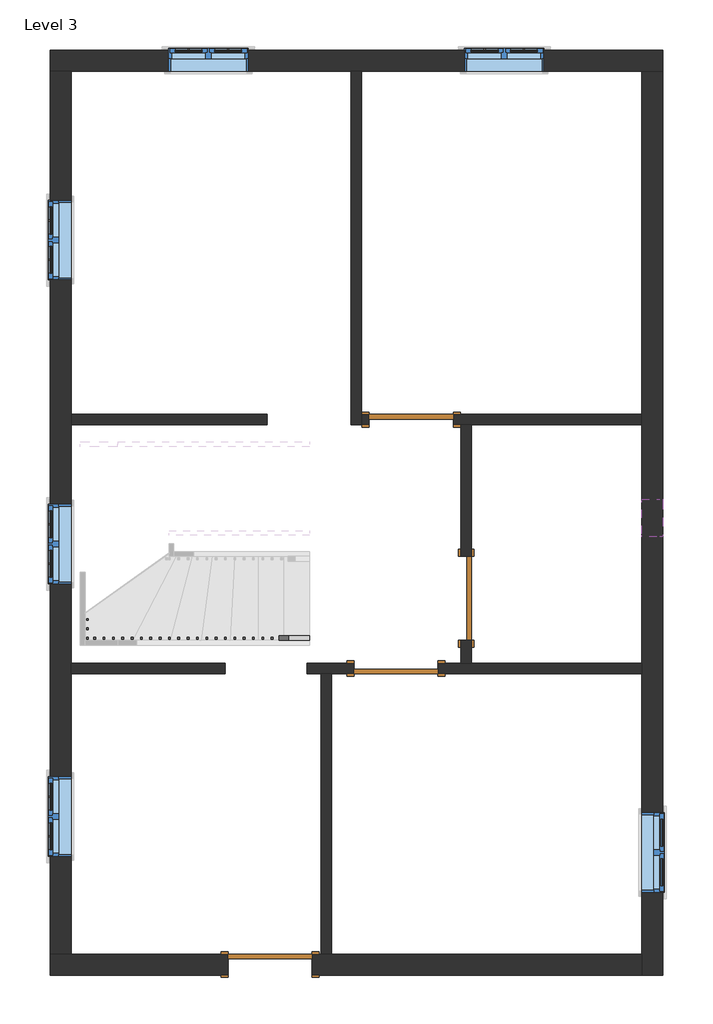
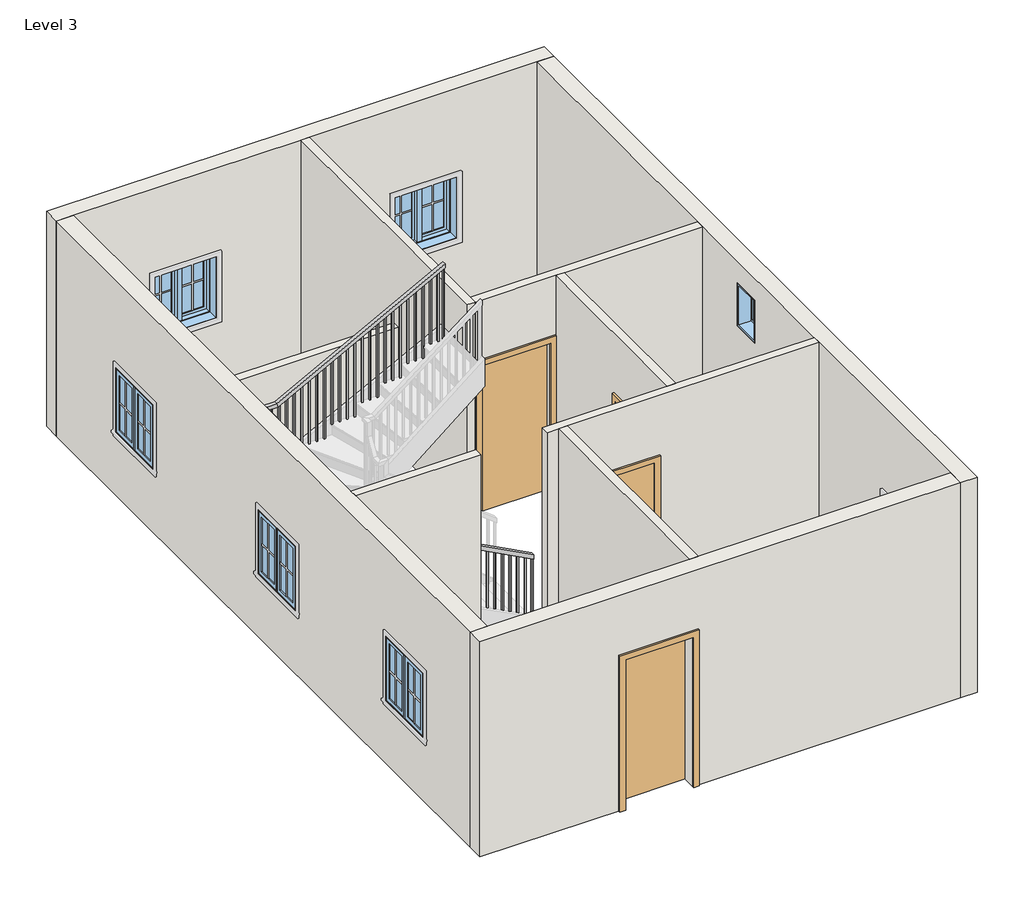
# One storey, part 1 of 2: 11 walls, 7 windows, 4 doors, 1 railing.
"""IFC4 building model written with IfcOpenShell, lengths in millimetres."""

from ifc_helpers import new_model, si_unit, frame, origin, place, context, project, spatial, polyline, outline, extrude, faceted_brep, transform, mapped, element, save
from components import door_e5f9f3c4, door_305aa2a5, door_a90ba1ad, window_aa618e30, window_339605e1

model = new_model("IFC4")

# Units and contexts
model_context = context("Model", 3, world=origin())
ifc_project = project(units=[si_unit("LENGTHUNIT", "METRE", prefix="MILLI")], contexts=[model_context])

# Site, building, storey
site = spatial("IfcSite", under=ifc_project)
building = spatial("IfcBuilding", under=site)
storey = spatial("IfcBuildingStorey", under=building, Name="Level 3", Elevation=3200.4)

# Doors
placement = place(None, origin())
door_shape = door_e5f9f3c4(model_context)
element("IfcDoor", 1, ObjectType="Single-Flush : 36\" x 84\"", at=placement, inside=storey, context=model_context, shape_type="MappedRepresentation", body=[
    mapped(door_shape, transform((-78.9949167, -802.9070853, 3200.4), x_axis=(0.0, -1.0, 0.0), y_axis=(1.0, 0.0, 0.0), z_axis=(0.0, 0.0, 1.0))),
])
element("IfcDoor", 2, ObjectType="Single-Flush : 36\" x 84\"", at=placement, inside=storey, context=model_context, shape_type="MappedRepresentation", body=[
    mapped(door_shape, transform((-840.9949167, -1564.9070853, 3200.4), x_axis=(-1.0, 0.0, 0.0), y_axis=(0.0, -1.0, 0.0), z_axis=(0.0, 0.0, 1.0))),
])
door_2_shape = door_305aa2a5(model_context)
element("IfcDoor", 3, ObjectType="Single-Flush : 36\" x 84\"", at=placement, inside=storey, context=model_context, shape_type="MappedRepresentation", body=[
    mapped(door_2_shape, transform((-675.8949167, 1140.1929147, 3200.4), x_axis=(-1.0, 0.0, 0.0), y_axis=(0.0, -1.0, 0.0), z_axis=(0.0, 0.0, 1.0))),
])
door_3_shape = door_a90ba1ad(model_context)
element("IfcDoor", 4, ObjectType="Single-Flush : 36\" x 84\"", at=placement, inside=storey, context=model_context, shape_type="MappedRepresentation", body=[
    mapped(door_3_shape, transform((-2212.5949167, -4784.3570853, 3200.4), x_axis=(-1.0, 0.0, 0.0), y_axis=(0.0, -1.0, 0.0), z_axis=(0.0, 0.0, 1.0))),
])

# Railing
element("IfcRailing", 5, ObjectType="Handrail - Rectangular", at=placement, inside=storey, context=model_context, shape_type="SolidModel", body=[
    faceted_brep([(-1783.4132248, -1260.1070853, 4284.1333333), (-1783.4132248, -1260.1070853, 4226.6742652), (-1783.4132248, -1209.3070853, 4226.6742652), (-1783.4132248, -1209.3070853, 4284.1333333), (-4041.1382869, -1260.1070853, 5477.4239201), (-4053.7373514, -1260.1070853, 5426.6239201), (-4053.7373514, -1209.3070853, 5426.6239201), (-4041.1382869, -1209.3070853, 5477.4239201), (-4225.5449167, -1260.1070853, 5477.4239201), (-4225.5449167, -1260.1070853, 5426.6239201), (-4174.7449167, -1209.3070853, 5426.6239201), (-4174.7449167, -1209.3070853, 5477.4239201), (-4225.5449167, -972.7952032, 5477.4239201), (-4225.5449167, -964.8446271, 5426.6239201), (-4174.7449167, -964.8446271, 5426.6239201), (-4174.7449167, -972.7952032, 5477.4239201), (-4225.5449167, 560.7810325, 5969.5094132), (-4225.5449167, 568.7316087, 5918.7094132), (-4174.7449167, 568.7316087, 5918.7094132), (-4174.7449167, 560.7810325, 5969.5094132), (-4225.5449167, 848.0929147, 5969.5094132), (-4225.5449167, 848.0929147, 5918.7094132), (-4174.7449167, 797.2929147, 5918.7094132), (-4174.7449167, 797.2929147, 5969.5094132), (-4041.1382869, 848.0929147, 5969.5094132), (-4028.5392223, 848.0929147, 5918.7094132), (-4028.5392223, 797.2929147, 5918.7094132), (-4041.1382869, 797.2929147, 5969.5094132), (-1783.4132248, 848.0929147, 7162.8), (-1783.4132248, 797.2929147, 7162.8), (-1783.4132248, 797.2929147, 7105.3409318), (-1783.4132248, 848.0929147, 7105.3409318)], [[[0, 1, 2, 3]], [[1, 0, 4, 5]], [[2, 1, 5, 6]], [[3, 2, 6, 7]], [[0, 3, 7, 4]], [[5, 4, 8, 9]], [[6, 5, 9, 10]], [[7, 6, 10, 11]], [[4, 7, 11, 8]], [[9, 8, 12, 13]], [[10, 9, 13, 14]], [[11, 10, 14, 15]], [[8, 11, 15, 12]], [[13, 12, 16, 17]], [[14, 13, 17, 18]], [[15, 14, 18, 19]], [[12, 15, 19, 16]], [[17, 16, 20, 21]], [[18, 17, 21, 22]], [[19, 18, 22, 23]], [[16, 19, 23, 20]], [[21, 20, 24, 25]], [[22, 21, 25, 26]], [[23, 22, 26, 27]], [[20, 23, 27, 24]], [[28, 29, 30, 31]], [[25, 24, 28, 31]], [[26, 25, 31, 30]], [[27, 26, 30, 29]], [[24, 27, 29, 28]]]),
    extrude(outline(polyline([(7058.0597858, -1872.8699167), (6079.0666667, -1872.8699167), (6079.0666667, -1853.8199167), (7068.1284102, -1853.8199167), (7058.0597858, -1872.8699167)])), frame((0.0, 813.1679147, 0.0), z_axis=(0.0, 1.0, 0.0), x_axis=(0.0, 0.0, 1.0)), (0.0, 0.0, 1.0), 19.05),
    extrude(outline(polyline([(7004.3604556, -1974.4699167), (6079.0666667, -1974.4699167), (6079.0666667, -1955.4199167), (7014.42908, -1955.4199167), (7004.3604556, -1974.4699167)])), frame((0.0, 813.1679147, 0.0), z_axis=(0.0, 1.0, 0.0), x_axis=(0.0, 0.0, 1.0)), (0.0, 0.0, 1.0), 19.05),
    extrude(outline(polyline([(6950.6611254, -2076.0699167), (5909.7333333, -2076.0699167), (5909.7333333, -2057.0199167), (6960.7297498, -2057.0199167), (6950.6611254, -2076.0699167)])), frame((0.0, 813.1679147, 0.0), z_axis=(0.0, 1.0, 0.0), x_axis=(0.0, 0.0, 1.0)), (0.0, 0.0, 1.0), 19.05),
    extrude(outline(polyline([(6896.9617952, -2177.6699167), (5909.7333333, -2177.6699167), (5909.7333333, -2158.6199167), (6907.0304196, -2158.6199167), (6896.9617952, -2177.6699167)])), frame((0.0, 813.1679147, 0.0), z_axis=(0.0, 1.0, 0.0), x_axis=(0.0, 0.0, 1.0)), (0.0, 0.0, 1.0), 19.05),
    extrude(outline(polyline([(6843.262465, -2279.2699167), (5909.7333333, -2279.2699167), (5909.7333333, -2260.2199167), (6853.3310894, -2260.2199167), (6843.262465, -2279.2699167)])), frame((0.0, 813.1679147, 0.0), z_axis=(0.0, 1.0, 0.0), x_axis=(0.0, 0.0, 1.0)), (0.0, 0.0, 1.0), 19.05),
    extrude(outline(polyline([(6789.5631348, -2380.8699167), (5740.4, -2380.8699167), (5740.4, -2361.8199167), (6799.6317592, -2361.8199167), (6789.5631348, -2380.8699167)])), frame((0.0, 813.1679147, 0.0), z_axis=(0.0, 1.0, 0.0), x_axis=(0.0, 0.0, 1.0)), (0.0, 0.0, 1.0), 19.05),
    extrude(outline(polyline([(6735.8638046, -2482.4699167), (5740.4, -2482.4699167), (5740.4, -2463.4199167), (6745.932429, -2463.4199167), (6735.8638046, -2482.4699167)])), frame((0.0, 813.1679147, 0.0), z_axis=(0.0, 1.0, 0.0), x_axis=(0.0, 0.0, 1.0)), (0.0, 0.0, 1.0), 19.05),
    extrude(outline(polyline([(6682.1644744, -2584.0699167), (5740.4, -2584.0699167), (5740.4, -2565.0199167), (6692.2330988, -2565.0199167), (6682.1644744, -2584.0699167)])), frame((0.0, 813.1679147, 0.0), z_axis=(0.0, 1.0, 0.0), x_axis=(0.0, 0.0, 1.0)), (0.0, 0.0, 1.0), 19.05),
    extrude(outline(polyline([(6628.4651442, -2685.6699167), (5571.0666667, -2685.6699167), (5571.0666667, -2666.6199167), (6638.5337686, -2666.6199167), (6628.4651442, -2685.6699167)])), frame((0.0, 813.1679147, 0.0), z_axis=(0.0, 1.0, 0.0), x_axis=(0.0, 0.0, 1.0)), (0.0, 0.0, 1.0), 19.05),
    extrude(outline(polyline([(6574.765814, -2787.2699167), (5571.0666667, -2787.2699167), (5571.0666667, -2768.2199167), (6584.8344384, -2768.2199167), (6574.765814, -2787.2699167)])), frame((0.0, 813.1679147, 0.0), z_axis=(0.0, 1.0, 0.0), x_axis=(0.0, 0.0, 1.0)), (0.0, 0.0, 1.0), 19.05),
    extrude(outline(polyline([(6521.0664838, -2888.8699167), (5571.0666667, -2888.8699167), (5571.0666667, -2869.8199167), (6531.1351082, -2869.8199167), (6521.0664838, -2888.8699167)])), frame((0.0, 813.1679147, 0.0), z_axis=(0.0, 1.0, 0.0), x_axis=(0.0, 0.0, 1.0)), (0.0, 0.0, 1.0), 19.05),
    extrude(outline(polyline([(6467.3671536, -2990.4699167), (5401.7333333, -2990.4699167), (5401.7333333, -2971.4199167), (6477.435778, -2971.4199167), (6467.3671536, -2990.4699167)])), frame((0.0, 813.1679147, 0.0), z_axis=(0.0, 1.0, 0.0), x_axis=(0.0, 0.0, 1.0)), (0.0, 0.0, 1.0), 19.05),
    extrude(outline(polyline([(6413.6678234, -3092.0699167), (5401.7333333, -3092.0699167), (5401.7333333, -3073.0199167), (6423.7364478, -3073.0199167), (6413.6678234, -3092.0699167)])), frame((0.0, 813.1679147, 0.0), z_axis=(0.0, 1.0, 0.0), x_axis=(0.0, 0.0, 1.0)), (0.0, 0.0, 1.0), 19.05),
    extrude(outline(polyline([(6359.9684932, -3193.6699167), (5401.7333333, -3193.6699167), (5401.7333333, -3174.6199167), (6370.0371176, -3174.6199167), (6359.9684932, -3193.6699167)])), frame((0.0, 813.1679147, 0.0), z_axis=(0.0, 1.0, 0.0), x_axis=(0.0, 0.0, 1.0)), (0.0, 0.0, 1.0), 19.05),
    extrude(outline(polyline([(6306.269163, -3295.2699167), (5401.7333333, -3295.2699167), (5401.7333333, -3276.2199167), (6316.3377874, -3276.2199167), (6306.269163, -3295.2699167)])), frame((0.0, 813.1679147, 0.0), z_axis=(0.0, 1.0, 0.0), x_axis=(0.0, 0.0, 1.0)), (0.0, 0.0, 1.0), 19.05),
    extrude(outline(polyline([(6252.5698328, -3396.8699167), (5232.4, -3396.8699167), (5232.4, -3377.8199167), (6262.6384572, -3377.8199167), (6252.5698328, -3396.8699167)])), frame((0.0, 813.1679147, 0.0), z_axis=(0.0, 1.0, 0.0), x_axis=(0.0, 0.0, 1.0)), (0.0, 0.0, 1.0), 19.05),
    extrude(outline(polyline([(6198.8705026, -3498.4699167), (5232.4, -3498.4699167), (5232.4, -3479.4199167), (6208.939127, -3479.4199167), (6198.8705026, -3498.4699167)])), frame((0.0, 813.1679147, 0.0), z_axis=(0.0, 1.0, 0.0), x_axis=(0.0, 0.0, 1.0)), (0.0, 0.0, 1.0), 19.05),
    extrude(outline(polyline([(6145.1711724, -3600.0699167), (5232.4, -3600.0699167), (5232.4, -3581.0199167), (6155.2397968, -3581.0199167), (6145.1711724, -3600.0699167)])), frame((0.0, 813.1679147, 0.0), z_axis=(0.0, 1.0, 0.0), x_axis=(0.0, 0.0, 1.0)), (0.0, 0.0, 1.0), 19.05),
    extrude(outline(polyline([(6091.4718422, -3701.6699167), (5232.4, -3701.6699167), (5232.4, -3682.6199167), (6101.5404666, -3682.6199167), (6091.4718422, -3701.6699167)])), frame((0.0, 813.1679147, 0.0), z_axis=(0.0, 1.0, 0.0), x_axis=(0.0, 0.0, 1.0)), (0.0, 0.0, 1.0), 19.05),
    extrude(outline(polyline([(6037.772512, -3803.2699167), (5063.0666667, -3803.2699167), (5063.0666667, -3784.2199167), (6047.8411364, -3784.2199167), (6037.772512, -3803.2699167)])), frame((0.0, 813.1679147, 0.0), z_axis=(0.0, 1.0, 0.0), x_axis=(0.0, 0.0, 1.0)), (0.0, 0.0, 1.0), 19.05),
    extrude(outline(polyline([(5984.0731818, -3904.8699167), (5063.0666667, -3904.8699167), (5063.0666667, -3885.8199167), (5994.1418062, -3885.8199167), (5984.0731818, -3904.8699167)])), frame((0.0, 813.1679147, 0.0), z_axis=(0.0, 1.0, 0.0), x_axis=(0.0, 0.0, 1.0)), (0.0, 0.0, 1.0), 19.05),
    extrude(outline(polyline([(5930.3738516, -4006.4699167), (5063.0666667, -4006.4699167), (5063.0666667, -3987.4199167), (5940.442476, -3987.4199167), (5930.3738516, -4006.4699167)])), frame((0.0, 813.1679147, 0.0), z_axis=(0.0, 1.0, 0.0), x_axis=(0.0, 0.0, 1.0)), (0.0, 0.0, 1.0), 19.05),
    extrude(outline(polyline([(-4108.0699167, 832.2179147), (-4089.0199167, 832.2179147), (-4089.0199167, 813.1679147), (-4108.0699167, 813.1679147), (-4108.0699167, 832.2179147)])), frame((0.0, 0.0, 5063.0666667), z_axis=(0.0, 0.0, 1.0), x_axis=(1.0, 0.0, 0.0)), (0.0, 0.0, 1.0), 855.6427466),
    extrude(outline(polyline([(-4209.6699167, 787.7679147), (-4209.6699167, 806.8179147), (-4190.6199167, 806.8179147), (-4190.6199167, 787.7679147), (-4209.6699167, 787.7679147)])), frame((0.0, 0.0, 5063.0666667), z_axis=(0.0, 0.0, 1.0), x_axis=(1.0, 0.0, 0.0)), (0.0, 0.0, 1.0), 855.6427466),
    extrude(outline(polyline([(-4209.6699167, 686.1679147), (-4209.6699167, 705.2179147), (-4190.6199167, 705.2179147), (-4190.6199167, 686.1679147), (-4209.6699167, 686.1679147)])), frame((0.0, 0.0, 5063.0666667), z_axis=(0.0, 0.0, 1.0), x_axis=(1.0, 0.0, 0.0)), (0.0, 0.0, 1.0), 855.6427466),
    extrude(outline(polyline([(-4209.6699167, 584.5679147), (-4209.6699167, 603.6179147), (-4190.6199167, 603.6179147), (-4190.6199167, 584.5679147), (-4209.6699167, 584.5679147)])), frame((0.0, 0.0, 5063.0666667), z_axis=(0.0, 0.0, 1.0), x_axis=(1.0, 0.0, 0.0)), (0.0, 0.0, 1.0), 855.6427466),
    extrude(outline(polyline([(502.0179147, 5897.3026907), (502.0179147, 4893.7333333), (482.9679147, 4893.7333333), (482.9679147, 5891.1900316), (502.0179147, 5897.3026907)])), frame((-4209.6699167, 0.0, 0.0), z_axis=(1.0, 0.0, 0.0), x_axis=(0.0, 1.0, 0.0)), (0.0, 0.0, 1.0), 19.05),
    extrude(outline(polyline([(400.4179147, 5864.7018425), (400.4179147, 4893.7333333), (381.3679147, 4893.7333333), (381.3679147, 5858.5891834), (400.4179147, 5864.7018425)])), frame((-4209.6699167, 0.0, 0.0), z_axis=(1.0, 0.0, 0.0), x_axis=(0.0, 1.0, 0.0)), (0.0, 0.0, 1.0), 19.05),
    extrude(outline(polyline([(298.8179147, 5832.1009942), (298.8179147, 4893.7333333), (279.7679147, 4893.7333333), (279.7679147, 5825.9883352), (298.8179147, 5832.1009942)])), frame((-4209.6699167, 0.0, 0.0), z_axis=(1.0, 0.0, 0.0), x_axis=(0.0, 1.0, 0.0)), (0.0, 0.0, 1.0), 19.05),
    extrude(outline(polyline([(197.2179147, 5799.500146), (197.2179147, 4893.7333333), (178.1679147, 4893.7333333), (178.1679147, 5793.387487), (197.2179147, 5799.500146)])), frame((-4209.6699167, 0.0, 0.0), z_axis=(1.0, 0.0, 0.0), x_axis=(0.0, 1.0, 0.0)), (0.0, 0.0, 1.0), 19.05),
    extrude(outline(polyline([(95.6179147, 5766.8992978), (95.6179147, 4893.7333333), (76.5679147, 4893.7333333), (76.5679147, 5760.7866387), (95.6179147, 5766.8992978)])), frame((-4209.6699167, 0.0, 0.0), z_axis=(1.0, 0.0, 0.0), x_axis=(0.0, 1.0, 0.0)), (0.0, 0.0, 1.0), 19.05),
    extrude(outline(polyline([(-5.9820853, 5734.2984495), (-5.9820853, 4724.4), (-25.0320853, 4724.4), (-25.0320853, 5728.1857905), (-5.9820853, 5734.2984495)])), frame((-4209.6699167, 0.0, 0.0), z_axis=(1.0, 0.0, 0.0), x_axis=(0.0, 1.0, 0.0)), (0.0, 0.0, 1.0), 19.05),
    extrude(outline(polyline([(-107.5820853, 5701.6976013), (-107.5820853, 4724.4), (-126.6320853, 4724.4), (-126.6320853, 5695.5849423), (-107.5820853, 5701.6976013)])), frame((-4209.6699167, 0.0, 0.0), z_axis=(1.0, 0.0, 0.0), x_axis=(0.0, 1.0, 0.0)), (0.0, 0.0, 1.0), 19.05),
    extrude(outline(polyline([(-209.1820853, 5669.0967531), (-209.1820853, 4724.4), (-228.2320853, 4724.4), (-228.2320853, 5662.984094), (-209.1820853, 5669.0967531)])), frame((-4209.6699167, 0.0, 0.0), z_axis=(1.0, 0.0, 0.0), x_axis=(0.0, 1.0, 0.0)), (0.0, 0.0, 1.0), 19.05),
    extrude(outline(polyline([(-310.7820853, 5636.4959049), (-310.7820853, 4724.4), (-329.8320853, 4724.4), (-329.8320853, 5630.3832458), (-310.7820853, 5636.4959049)])), frame((-4209.6699167, 0.0, 0.0), z_axis=(1.0, 0.0, 0.0), x_axis=(0.0, 1.0, 0.0)), (0.0, 0.0, 1.0), 19.05),
    extrude(outline(polyline([(-412.3820853, 5603.8950566), (-412.3820853, 4724.4), (-431.4320853, 4724.4), (-431.4320853, 5597.7823976), (-412.3820853, 5603.8950566)])), frame((-4209.6699167, 0.0, 0.0), z_axis=(1.0, 0.0, 0.0), x_axis=(0.0, 1.0, 0.0)), (0.0, 0.0, 1.0), 19.05),
    extrude(outline(polyline([(-513.9820853, 5571.2942084), (-513.9820853, 4555.0666667), (-533.0320853, 4555.0666667), (-533.0320853, 5565.1815494), (-513.9820853, 5571.2942084)])), frame((-4209.6699167, 0.0, 0.0), z_axis=(1.0, 0.0, 0.0), x_axis=(0.0, 1.0, 0.0)), (0.0, 0.0, 1.0), 19.05),
    extrude(outline(polyline([(-615.5820853, 5538.6933602), (-615.5820853, 4555.0666667), (-634.6320853, 4555.0666667), (-634.6320853, 5532.5807011), (-615.5820853, 5538.6933602)])), frame((-4209.6699167, 0.0, 0.0), z_axis=(1.0, 0.0, 0.0), x_axis=(0.0, 1.0, 0.0)), (0.0, 0.0, 1.0), 19.05),
    extrude(outline(polyline([(-717.1820853, 5506.092512), (-717.1820853, 4555.0666667), (-736.2320853, 4555.0666667), (-736.2320853, 5499.9798529), (-717.1820853, 5506.092512)])), frame((-4209.6699167, 0.0, 0.0), z_axis=(1.0, 0.0, 0.0), x_axis=(0.0, 1.0, 0.0)), (0.0, 0.0, 1.0), 19.05),
    extrude(outline(polyline([(-818.7820853, 5473.4916637), (-818.7820853, 4555.0666667), (-837.8320853, 4555.0666667), (-837.8320853, 5467.3790047), (-818.7820853, 5473.4916637)])), frame((-4209.6699167, 0.0, 0.0), z_axis=(1.0, 0.0, 0.0), x_axis=(0.0, 1.0, 0.0)), (0.0, 0.0, 1.0), 19.05),
    extrude(outline(polyline([(-920.3820853, 5440.8908155), (-920.3820853, 4555.0666667), (-939.4320853, 4555.0666667), (-939.4320853, 5434.7781565), (-920.3820853, 5440.8908155)])), frame((-4209.6699167, 0.0, 0.0), z_axis=(1.0, 0.0, 0.0), x_axis=(0.0, 1.0, 0.0)), (0.0, 0.0, 1.0), 19.05),
    extrude(outline(polyline([(-4209.6699167, -1041.0320853), (-4209.6699167, -1021.9820853), (-4190.6199167, -1021.9820853), (-4190.6199167, -1041.0320853), (-4209.6699167, -1041.0320853)])), frame((0.0, 0.0, 4385.7333333), z_axis=(0.0, 0.0, 1.0), x_axis=(1.0, 0.0, 0.0)), (0.0, 0.0, 1.0), 1040.8905868),
    extrude(outline(polyline([(-4209.6699167, -1142.6320853), (-4209.6699167, -1123.5820853), (-4190.6199167, -1123.5820853), (-4190.6199167, -1142.6320853), (-4209.6699167, -1142.6320853)])), frame((0.0, 0.0, 4385.7333333), z_axis=(0.0, 0.0, 1.0), x_axis=(1.0, 0.0, 0.0)), (0.0, 0.0, 1.0), 1040.8905868),
    extrude(outline(polyline([(-4110.6882248, -1244.2320853), (-4129.7382248, -1244.2320853), (-4129.7382248, -1225.1820853), (-4110.6882248, -1225.1820853), (-4110.6882248, -1244.2320853)])), frame((0.0, 0.0, 4385.7333333), z_axis=(0.0, 0.0, 1.0), x_axis=(1.0, 0.0, 0.0)), (0.0, 0.0, 1.0), 1040.8905868),
    extrude(outline(polyline([(5413.0938418, -4028.1382248), (4385.7333333, -4028.1382248), (4385.7333333, -4009.0882248), (5403.0252174, -4009.0882248), (5413.0938418, -4028.1382248)])), frame((0.0, -1244.2320853, 0.0), z_axis=(0.0, 1.0, 0.0), x_axis=(0.0, 0.0, 1.0)), (0.0, 0.0, 1.0), 19.05),
    extrude(outline(polyline([(5359.3945116, -3926.5382248), (4385.7333333, -3926.5382248), (4385.7333333, -3907.4882248), (5349.3258872, -3907.4882248), (5359.3945116, -3926.5382248)])), frame((0.0, -1244.2320853, 0.0), z_axis=(0.0, 1.0, 0.0), x_axis=(0.0, 0.0, 1.0)), (0.0, 0.0, 1.0), 19.05),
    extrude(outline(polyline([(5305.6951814, -3824.9382248), (4385.7333333, -3824.9382248), (4385.7333333, -3805.8882248), (5295.626557, -3805.8882248), (5305.6951814, -3824.9382248)])), frame((0.0, -1244.2320853, 0.0), z_axis=(0.0, 1.0, 0.0), x_axis=(0.0, 0.0, 1.0)), (0.0, 0.0, 1.0), 19.05),
    extrude(outline(polyline([(5251.9958512, -3723.3382248), (4385.7333333, -3723.3382248), (4385.7333333, -3704.2882248), (5241.9272268, -3704.2882248), (5251.9958512, -3723.3382248)])), frame((0.0, -1244.2320853, 0.0), z_axis=(0.0, 1.0, 0.0), x_axis=(0.0, 0.0, 1.0)), (0.0, 0.0, 1.0), 19.05),
    extrude(outline(polyline([(5198.296521, -3621.7382248), (4216.4, -3621.7382248), (4216.4, -3602.6882248), (5188.2278966, -3602.6882248), (5198.296521, -3621.7382248)])), frame((0.0, -1244.2320853, 0.0), z_axis=(0.0, 1.0, 0.0), x_axis=(0.0, 0.0, 1.0)), (0.0, 0.0, 1.0), 19.05),
    extrude(outline(polyline([(5144.5971908, -3520.1382248), (4216.4, -3520.1382248), (4216.4, -3501.0882248), (5134.5285664, -3501.0882248), (5144.5971908, -3520.1382248)])), frame((0.0, -1244.2320853, 0.0), z_axis=(0.0, 1.0, 0.0), x_axis=(0.0, 0.0, 1.0)), (0.0, 0.0, 1.0), 19.05),
    extrude(outline(polyline([(5090.8978606, -3418.5382248), (4216.4, -3418.5382248), (4216.4, -3399.4882248), (5080.8292362, -3399.4882248), (5090.8978606, -3418.5382248)])), frame((0.0, -1244.2320853, 0.0), z_axis=(0.0, 1.0, 0.0), x_axis=(0.0, 0.0, 1.0)), (0.0, 0.0, 1.0), 19.05),
    extrude(outline(polyline([(5037.1985304, -3316.9382248), (4216.4, -3316.9382248), (4216.4, -3297.8882248), (5027.129906, -3297.8882248), (5037.1985304, -3316.9382248)])), frame((0.0, -1244.2320853, 0.0), z_axis=(0.0, 1.0, 0.0), x_axis=(0.0, 0.0, 1.0)), (0.0, 0.0, 1.0), 19.05),
    extrude(outline(polyline([(4983.4992002, -3215.3382248), (4047.0666667, -3215.3382248), (4047.0666667, -3196.2882248), (4973.4305758, -3196.2882248), (4983.4992002, -3215.3382248)])), frame((0.0, -1244.2320853, 0.0), z_axis=(0.0, 1.0, 0.0), x_axis=(0.0, 0.0, 1.0)), (0.0, 0.0, 1.0), 19.05),
    extrude(outline(polyline([(4929.79987, -3113.7382248), (4047.0666667, -3113.7382248), (4047.0666667, -3094.6882248), (4919.7312456, -3094.6882248), (4929.79987, -3113.7382248)])), frame((0.0, -1244.2320853, 0.0), z_axis=(0.0, 1.0, 0.0), x_axis=(0.0, 0.0, 1.0)), (0.0, 0.0, 1.0), 19.05),
    extrude(outline(polyline([(4876.1005398, -3012.1382248), (4047.0666667, -3012.1382248), (4047.0666667, -2993.0882248), (4866.0319154, -2993.0882248), (4876.1005398, -3012.1382248)])), frame((0.0, -1244.2320853, 0.0), z_axis=(0.0, 1.0, 0.0), x_axis=(0.0, 0.0, 1.0)), (0.0, 0.0, 1.0), 19.05),
    extrude(outline(polyline([(4822.4012096, -2910.5382248), (3877.7333333, -2910.5382248), (3877.7333333, -2891.4882248), (4812.3325852, -2891.4882248), (4822.4012096, -2910.5382248)])), frame((0.0, -1244.2320853, 0.0), z_axis=(0.0, 1.0, 0.0), x_axis=(0.0, 0.0, 1.0)), (0.0, 0.0, 1.0), 19.05),
    extrude(outline(polyline([(4768.7018794, -2808.9382248), (3877.7333333, -2808.9382248), (3877.7333333, -2789.8882248), (4758.633255, -2789.8882248), (4768.7018794, -2808.9382248)])), frame((0.0, -1244.2320853, 0.0), z_axis=(0.0, 1.0, 0.0), x_axis=(0.0, 0.0, 1.0)), (0.0, 0.0, 1.0), 19.05),
    extrude(outline(polyline([(4715.0025492, -2707.3382248), (3877.7333333, -2707.3382248), (3877.7333333, -2688.2882248), (4704.9339248, -2688.2882248), (4715.0025492, -2707.3382248)])), frame((0.0, -1244.2320853, 0.0), z_axis=(0.0, 1.0, 0.0), x_axis=(0.0, 0.0, 1.0)), (0.0, 0.0, 1.0), 19.05),
    extrude(outline(polyline([(4661.303219, -2605.7382248), (3708.4, -2605.7382248), (3708.4, -2586.6882248), (4651.2345946, -2586.6882248), (4661.303219, -2605.7382248)])), frame((0.0, -1244.2320853, 0.0), z_axis=(0.0, 1.0, 0.0), x_axis=(0.0, 0.0, 1.0)), (0.0, 0.0, 1.0), 19.05),
    extrude(outline(polyline([(4607.6038888, -2504.1382248), (3708.4, -2504.1382248), (3708.4, -2485.0882248), (4597.5352644, -2485.0882248), (4607.6038888, -2504.1382248)])), frame((0.0, -1244.2320853, 0.0), z_axis=(0.0, 1.0, 0.0), x_axis=(0.0, 0.0, 1.0)), (0.0, 0.0, 1.0), 19.05),
    extrude(outline(polyline([(4553.9045586, -2402.5382248), (3708.4, -2402.5382248), (3708.4, -2383.4882248), (4543.8359342, -2383.4882248), (4553.9045586, -2402.5382248)])), frame((0.0, -1244.2320853, 0.0), z_axis=(0.0, 1.0, 0.0), x_axis=(0.0, 0.0, 1.0)), (0.0, 0.0, 1.0), 19.05),
    extrude(outline(polyline([(4500.2052284, -2300.9382248), (3539.0666667, -2300.9382248), (3539.0666667, -2281.8882248), (4490.136604, -2281.8882248), (4500.2052284, -2300.9382248)])), frame((0.0, -1244.2320853, 0.0), z_axis=(0.0, 1.0, 0.0), x_axis=(0.0, 0.0, 1.0)), (0.0, 0.0, 1.0), 19.05),
    extrude(outline(polyline([(4446.5058982, -2199.3382248), (3539.0666667, -2199.3382248), (3539.0666667, -2180.2882248), (4436.4372738, -2180.2882248), (4446.5058982, -2199.3382248)])), frame((0.0, -1244.2320853, 0.0), z_axis=(0.0, 1.0, 0.0), x_axis=(0.0, 0.0, 1.0)), (0.0, 0.0, 1.0), 19.05),
    extrude(outline(polyline([(4392.806568, -2097.7382248), (3539.0666667, -2097.7382248), (3539.0666667, -2078.6882248), (4382.7379436, -2078.6882248), (4392.806568, -2097.7382248)])), frame((0.0, -1244.2320853, 0.0), z_axis=(0.0, 1.0, 0.0), x_axis=(0.0, 0.0, 1.0)), (0.0, 0.0, 1.0), 19.05),
    extrude(outline(polyline([(4339.1072378, -1996.1382248), (3369.7333333, -1996.1382248), (3369.7333333, -1977.0882248), (4329.0386134, -1977.0882248), (4339.1072378, -1996.1382248)])), frame((0.0, -1244.2320853, 0.0), z_axis=(0.0, 1.0, 0.0), x_axis=(0.0, 0.0, 1.0)), (0.0, 0.0, 1.0), 19.05),
    extrude(outline(polyline([(4285.4079076, -1894.5382248), (3369.7333333, -1894.5382248), (3369.7333333, -1875.4882248), (4275.3392831, -1875.4882248), (4285.4079076, -1894.5382248)])), frame((0.0, -1244.2320853, 0.0), z_axis=(0.0, 1.0, 0.0), x_axis=(0.0, 0.0, 1.0)), (0.0, 0.0, 1.0), 19.05),
    extrude(outline(polyline([(-4209.6699167, 813.1679147), (-4209.6699167, 832.2179147), (-4190.6199167, 832.2179147), (-4190.6199167, 813.1679147), (-4209.6699167, 813.1679147)])), frame((0.0, 0.0, 5063.0666667), z_axis=(0.0, 0.0, 1.0), x_axis=(1.0, 0.0, 0.0)), (0.0, 0.0, 1.0), 855.6427466),
    extrude(outline(polyline([(-4190.6199167, -1244.2320853), (-4209.6699167, -1244.2320853), (-4209.6699167, -1225.1820853), (-4190.6199167, -1225.1820853), (-4190.6199167, -1244.2320853)])), frame((0.0, 0.0, 4385.7333333), z_axis=(0.0, 0.0, 1.0), x_axis=(1.0, 0.0, 0.0)), (0.0, 0.0, 1.0), 1040.8905868),
    extrude(outline(polyline([(7095.2723074, -1802.4632248), (6079.0666667, -1802.4632248), (6079.0666667, -1783.4132248), (7105.3409318, -1783.4132248), (7095.2723074, -1802.4632248)])), frame((0.0, 813.1679147, 0.0), z_axis=(0.0, 1.0, 0.0), x_axis=(0.0, 0.0, 1.0)), (0.0, 0.0, 1.0), 19.05),
    extrude(outline(polyline([(4236.7428896, -1802.4632248), (3369.7333333, -1802.4632248), (3369.7333333, -1783.4132248), (4226.6742652, -1783.4132248), (4236.7428896, -1802.4632248)])), frame((0.0, -1244.2320853, 0.0), z_axis=(0.0, 1.0, 0.0), x_axis=(0.0, 0.0, 1.0)), (0.0, 0.0, 1.0), 19.05),
])

# Walls
element("IfcWall", 6, ObjectType="WALL4.5\"", at=placement, inside=storey, context=model_context, shape_type="Brep", body=[
    faceted_brep([(-1329.9449167, 4931.1429147, 3200.4), (-1329.9449167, 1083.0429147, 3200.4), (-1329.9449167, 1083.0429147, 6248.4), (-1329.9449167, 4931.1429147, 6248.4), (-1215.6449167, 4931.1429147, 3200.4), (-1215.6449167, 4931.1429147, 6248.4), (-1215.6449167, 1197.3429147, 6248.4), (-1215.6449167, 1083.0429147, 6248.4), (-1215.6449167, 1083.0429147, 3200.4), (-1215.6449167, 1197.3429147, 3200.4)], [[[0, 1, 2, 3]], [[4, 5, 6, 7, 8, 9]], [[1, 0, 4, 9, 8]], [[0, 3, 5, 4]], [[2, 1, 8, 7]], [[3, 2, 7, 6, 5]]]),
])
element("IfcWall", 7, ObjectType="WALL4.5\"", at=placement, inside=storey, context=model_context, shape_type="Brep", body=[
    faceted_brep([(-1215.6449167, 1083.0429147, 3200.4), (-1133.0949167, 1083.0429147, 3200.4), (-1133.0949167, 1083.0429147, 5334.0), (-218.6949167, 1083.0429147, 5334.0), (-218.6949167, 1083.0429147, 3200.4), (-136.1449167, 1083.0429147, 3200.4), (-21.8449167, 1083.0429147, 3200.4), (1832.3550833, 1083.0429147, 3200.4), (1832.3550833, 1083.0429147, 6248.4), (-21.8449167, 1083.0429147, 6248.4), (-136.1449167, 1083.0429147, 6248.4), (-1215.6449167, 1083.0429147, 6248.4), (-1133.0949167, 1197.3429147, 5334.0), (-1133.0949167, 1197.3429147, 3200.4), (-1215.6449167, 1197.3429147, 3200.4), (-1215.6449167, 1197.3429147, 6248.4), (1832.3550833, 1197.3429147, 6248.4), (1832.3550833, 1197.3429147, 3200.4), (-218.6949167, 1197.3429147, 3200.4), (-218.6949167, 1197.3429147, 5334.0)], [[[0, 1, 2, 3, 4, 5, 6, 7, 8, 9, 10, 11]], [[12, 13, 14, 15, 16, 17, 18, 19]], [[18, 17, 7, 6, 5, 4]], [[14, 13, 1, 0]], [[0, 11, 15, 14]], [[8, 7, 17, 16]], [[2, 1, 13, 12]], [[3, 2, 12, 19]], [[4, 3, 19, 18]], [[11, 10, 9, 8, 16, 15]]]),
])
element("IfcWall", 8, ObjectType="WALL4.5\"", at=placement, inside=storey, context=model_context, shape_type="SweptSolid", body=[
    extrude(outline(polyline([(-2244.3449167, 1083.0429147), (-4377.9449167, 1083.0429147), (-4377.9449167, 1197.3429147), (-2244.3449167, 1197.3429147), (-2244.3449167, 1083.0429147)])), frame((0.0, 0.0, 3200.4), z_axis=(0.0, 0.0, 1.0), x_axis=(1.0, 0.0, 0.0)), (0.0, 0.0, 1.0), 3048.0),
])
element("IfcWall", 9, ObjectType="WALL4.5\"", at=placement, inside=storey, context=model_context, shape_type="SweptSolid", body=[
    extrude(outline(polyline([(-1260.1070853, 5334.0), (-1260.1070853, 3200.4), (-1507.7570853, 3200.4), (-1507.7570853, 6248.4), (1083.0429147, 6248.4), (1083.0429147, 3200.4), (-345.7070853, 3200.4), (-345.7070853, 5334.0), (-1260.1070853, 5334.0)])), frame((-136.1449167, 0.0, 0.0), z_axis=(1.0, 0.0, 0.0), x_axis=(0.0, 1.0, 0.0)), (0.0, 0.0, 1.0), 114.3),
])
element("IfcWall", 10, ObjectType="WALL4.5\"", at=placement, inside=storey, context=model_context, shape_type="SweptSolid", body=[
    extrude(outline(polyline([(-2701.5449167, -1622.0570853), (-4377.9449167, -1622.0570853), (-4377.9449167, -1507.7570853), (-2701.5449167, -1507.7570853), (-2701.5449167, -1622.0570853)])), frame((0.0, 0.0, 3200.4), z_axis=(0.0, 0.0, 1.0), x_axis=(1.0, 0.0, 0.0)), (0.0, 0.0, 1.0), 3048.0),
])
element("IfcWall", 11, ObjectType="WALL4.5\"", at=placement, inside=storey, context=model_context, shape_type="Brep", body=[
    faceted_brep([(-1812.5449167, -1622.0570853, 3200.4), (-1660.1449167, -1622.0570853, 3200.4), (-1545.8449167, -1622.0570853, 3200.4), (-1298.1949167, -1622.0570853, 3200.4), (-1298.1949167, -1622.0570853, 5334.0), (-383.7949167, -1622.0570853, 5334.0), (-383.7949167, -1622.0570853, 3200.4), (1832.3550833, -1622.0570853, 3200.4), (1832.3550833, -1622.0570853, 6248.4), (-1545.8449167, -1622.0570853, 6248.4), (-1660.1449167, -1622.0570853, 6248.4), (-1812.5449167, -1622.0570853, 6248.4), (-1298.1949167, -1507.7570853, 5334.0), (-1298.1949167, -1507.7570853, 3200.4), (-1812.5449167, -1507.7570853, 3200.4), (-1812.5449167, -1507.7570853, 6248.4), (-136.1449167, -1507.7570853, 6248.4), (-21.8449167, -1507.7570853, 6248.4), (1832.3550833, -1507.7570853, 6248.4), (1832.3550833, -1507.7570853, 3200.4), (-21.8449167, -1507.7570853, 3200.4), (-136.1449167, -1507.7570853, 3200.4), (-383.7949167, -1507.7570853, 3200.4), (-383.7949167, -1507.7570853, 5334.0)], [[[0, 1, 2, 3, 4, 5, 6, 7, 8, 9, 10, 11]], [[12, 13, 14, 15, 16, 17, 18, 19, 20, 21, 22, 23]], [[14, 13, 3, 2, 1, 0]], [[22, 21, 20, 19, 7, 6]], [[0, 11, 15, 14]], [[8, 7, 19, 18]], [[4, 3, 13, 12]], [[5, 4, 12, 23]], [[6, 5, 23, 22]], [[11, 10, 9, 8, 18, 17, 16, 15]]]),
])
element("IfcWall", 12, ObjectType="WALL4.5\"", at=placement, inside=storey, context=model_context, shape_type="SweptSolid", body=[
    extrude(outline(polyline([(-1660.1449167, -4670.0570853), (-1660.1449167, -1622.0570853), (-1545.8449167, -1622.0570853), (-1545.8449167, -4670.0570853), (-1660.1449167, -4670.0570853)])), frame((0.0, 0.0, 3200.4), z_axis=(0.0, 0.0, 1.0), x_axis=(1.0, 0.0, 0.0)), (0.0, 0.0, 1.0), 3048.0),
])
element("IfcWall", 13, ObjectType="WALL9\"", at=placement, inside=storey, context=model_context, shape_type="Brep", body=[
    faceted_brep([(-4606.5449167, 4931.1429147, 3200.4), (-4377.9449167, 4931.1429147, 3200.4), (-1329.9449167, 4931.1429147, 3200.4), (-1215.6449167, 4931.1429147, 3200.4), (1832.3550833, 4931.1429147, 3200.4), (2060.9550833, 4931.1429147, 3200.4), (2060.9550833, 4931.1429147, 6248.4), (1832.3550833, 4931.1429147, 6248.4), (-1215.6449167, 4931.1429147, 6248.4), (-1329.9449167, 4931.1429147, 6248.4), (-4377.9449167, 4931.1429147, 6248.4), (-4606.5449167, 4931.1429147, 6248.4), (-2450.7199167, 4931.1429147, 5029.2), (-2450.7199167, 4931.1429147, 4114.8), (-3314.3199167, 4931.1429147, 4114.8), (-3314.3199167, 4931.1429147, 5029.2), (768.7300833, 4931.1429147, 5029.2), (768.7300833, 4931.1429147, 4114.8), (-94.8699167, 4931.1429147, 4114.8), (-94.8699167, 4931.1429147, 5029.2), (-4606.5449167, 5159.7429147, 3200.4), (-4606.5449167, 5159.7429147, 6248.4), (2060.9550833, 5159.7429147, 6248.4), (2060.9550833, 5159.7429147, 3200.4), (-2450.7199167, 5159.7429147, 5029.2), (-3314.3199167, 5159.7429147, 5029.2), (-3314.3199167, 5159.7429147, 4114.8), (-2450.7199167, 5159.7429147, 4114.8), (768.7300833, 5159.7429147, 5029.2), (-94.8699167, 5159.7429147, 5029.2), (-94.8699167, 5159.7429147, 4114.8), (768.7300833, 5159.7429147, 4114.8)], [[[0, 1, 2, 3, 4, 5, 6, 7, 8, 9, 10, 11], [12, 13, 14, 15], [16, 17, 18, 19]], [[20, 21, 22, 23], [24, 25, 26, 27], [28, 29, 30, 31]], [[5, 4, 3, 2, 1, 0, 20, 23]], [[6, 5, 23, 22]], [[0, 11, 21, 20]], [[11, 10, 9, 8, 7, 6, 22, 21]], [[13, 12, 24, 27]], [[14, 13, 27, 26]], [[15, 14, 26, 25]], [[12, 15, 25, 24]], [[17, 16, 28, 31]], [[18, 17, 31, 30]], [[19, 18, 30, 29]], [[16, 19, 29, 28]]]),
])
element("IfcWall", 14, ObjectType="WALL9\"", at=placement, inside=storey, context=model_context, shape_type="Brep", body=[
    faceted_brep([(1832.3550833, 4931.1429147, 3200.4), (1832.3550833, 1197.3429147, 3200.4), (1832.3550833, 1083.0429147, 3200.4), (1832.3550833, -1507.7570853, 3200.4), (1832.3550833, -1622.0570853, 3200.4), (1832.3550833, -4670.0570853, 3200.4), (1832.3550833, -4898.6570853, 3200.4), (1832.3550833, -4898.6570853, 6248.4), (1832.3550833, -4670.0570853, 6248.4), (1832.3550833, -1622.0570853, 6248.4), (1832.3550833, -1507.7570853, 6248.4), (1832.3550833, 1083.0429147, 6248.4), (1832.3550833, 1197.3429147, 6248.4), (1832.3550833, 4931.1429147, 6248.4), (1832.3550833, -129.8070853, 5943.6), (1832.3550833, -129.8070853, 5334.0), (1832.3550833, 276.5929147, 5334.0), (1832.3550833, 276.5929147, 5943.6), (1832.3550833, -3996.9570853, 5029.2), (1832.3550833, -3996.9570853, 4114.8), (1832.3550833, -3133.3570853, 4114.8), (1832.3550833, -3133.3570853, 5029.2), (2060.9550833, 4931.1429147, 3200.4), (2060.9550833, 4931.1429147, 6248.4), (2060.9550833, -4898.6570853, 6248.4), (2060.9550833, -4898.6570853, 3200.4), (2060.9550833, -129.8070853, 5943.6), (2060.9550833, 276.5929147, 5943.6), (2060.9550833, 276.5929147, 5334.0), (2060.9550833, -129.8070853, 5334.0), (2060.9550833, -3996.9570853, 5029.2), (2060.9550833, -3133.3570853, 5029.2), (2060.9550833, -3133.3570853, 4114.8), (2060.9550833, -3996.9570853, 4114.8)], [[[0, 1, 2, 3, 4, 5, 6, 7, 8, 9, 10, 11, 12, 13], [14, 15, 16, 17], [18, 19, 20, 21]], [[22, 23, 24, 25], [26, 27, 28, 29], [30, 31, 32, 33]], [[6, 5, 4, 3, 2, 1, 0, 22, 25]], [[0, 13, 23, 22]], [[7, 6, 25, 24]], [[13, 12, 11, 10, 9, 8, 7, 24, 23]], [[15, 14, 26, 29]], [[16, 15, 29, 28]], [[17, 16, 28, 27]], [[14, 17, 27, 26]], [[19, 18, 30, 33]], [[20, 19, 33, 32]], [[21, 20, 32, 31]], [[18, 21, 31, 30]]]),
])
element("IfcWall", 15, ObjectType="WALL9\"", at=placement, inside=storey, context=model_context, shape_type="Brep", body=[
    faceted_brep([(-2669.7949167, -4670.0570853, 5334.0), (-2669.7949167, -4670.0570853, 3200.4), (-4377.9449167, -4670.0570853, 3200.4), (-4606.5449167, -4670.0570853, 3200.4), (-4606.5449167, -4670.0570853, 6248.4), (-4377.9449167, -4670.0570853, 6248.4), (-1660.1449167, -4670.0570853, 6248.4), (-1545.8449167, -4670.0570853, 6248.4), (1832.3550833, -4670.0570853, 6248.4), (1832.3550833, -4670.0570853, 3200.4), (-1545.8449167, -4670.0570853, 3200.4), (-1660.1449167, -4670.0570853, 3200.4), (-1755.3949167, -4670.0570853, 3200.4), (-1755.3949167, -4670.0570853, 5334.0), (-4606.5449167, -4898.6570853, 3200.4), (-2669.7949167, -4898.6570853, 3200.4), (-2669.7949167, -4898.6570853, 5334.0), (-1755.3949167, -4898.6570853, 5334.0), (-1755.3949167, -4898.6570853, 3200.4), (1832.3550833, -4898.6570853, 3200.4), (1832.3550833, -4898.6570853, 6248.4), (-4606.5449167, -4898.6570853, 6248.4)], [[[0, 1, 2, 3, 4, 5, 6, 7, 8, 9, 10, 11, 12, 13]], [[14, 15, 16, 17, 18, 19, 20, 21]], [[3, 2, 1, 15, 14]], [[12, 11, 10, 9, 19, 18]], [[9, 8, 20, 19]], [[4, 3, 14, 21]], [[16, 15, 1, 0]], [[17, 16, 0, 13]], [[18, 17, 13, 12]], [[8, 7, 6, 5, 4, 21, 20]]]),
])
element("IfcWall", 16, ObjectType="WALL9\"", at=placement, inside=storey, context=model_context, shape_type="Brep", body=[
    faceted_brep([(-4377.9449167, -4670.0570853, 3200.4), (-4377.9449167, -1622.0570853, 3200.4), (-4377.9449167, -1507.7570853, 3200.4), (-4377.9449167, 1083.0429147, 3200.4), (-4377.9449167, 1197.3429147, 3200.4), (-4377.9449167, 4931.1429147, 3200.4), (-4377.9449167, 4931.1429147, 6248.4), (-4377.9449167, 1197.3429147, 6248.4), (-4377.9449167, 1083.0429147, 6248.4), (-4377.9449167, -1507.7570853, 6248.4), (-4377.9449167, -1622.0570853, 6248.4), (-4377.9449167, -4670.0570853, 6248.4), (-4377.9449167, 219.4429147, 5029.2), (-4377.9449167, 219.4429147, 4114.8), (-4377.9449167, -644.1570853, 4114.8), (-4377.9449167, -644.1570853, 5029.2), (-4377.9449167, -2742.8320853, 5029.2), (-4377.9449167, -2742.8320853, 4114.8), (-4377.9449167, -3606.4320853, 4114.8), (-4377.9449167, -3606.4320853, 5029.2), (-4377.9449167, 3524.6179147, 5029.2), (-4377.9449167, 3524.6179147, 4114.8), (-4377.9449167, 2661.0179147, 4114.8), (-4377.9449167, 2661.0179147, 5029.2), (-4606.5449167, -4670.0570853, 3200.4), (-4606.5449167, -4670.0570853, 6248.4), (-4606.5449167, 4931.1429147, 6248.4), (-4606.5449167, 4931.1429147, 3200.4), (-4606.5449167, 219.4429147, 5029.2), (-4606.5449167, -644.1570853, 5029.2), (-4606.5449167, -644.1570853, 4114.8), (-4606.5449167, 219.4429147, 4114.8), (-4606.5449167, -2742.8320853, 5029.2), (-4606.5449167, -3606.4320853, 5029.2), (-4606.5449167, -3606.4320853, 4114.8), (-4606.5449167, -2742.8320853, 4114.8), (-4606.5449167, 3524.6179147, 5029.2), (-4606.5449167, 2661.0179147, 5029.2), (-4606.5449167, 2661.0179147, 4114.8), (-4606.5449167, 3524.6179147, 4114.8)], [[[0, 1, 2, 3, 4, 5, 6, 7, 8, 9, 10, 11], [12, 13, 14, 15], [16, 17, 18, 19], [20, 21, 22, 23]], [[24, 25, 26, 27], [28, 29, 30, 31], [32, 33, 34, 35], [36, 37, 38, 39]], [[5, 4, 3, 2, 1, 0, 24, 27]], [[0, 11, 25, 24]], [[6, 5, 27, 26]], [[11, 10, 9, 8, 7, 6, 26, 25]], [[13, 12, 28, 31]], [[14, 13, 31, 30]], [[15, 14, 30, 29]], [[12, 15, 29, 28]], [[17, 16, 32, 35]], [[18, 17, 35, 34]], [[19, 18, 34, 33]], [[16, 19, 33, 32]], [[21, 20, 36, 39]], [[22, 21, 39, 38]], [[23, 22, 38, 37]], [[20, 23, 37, 36]]]),
])

# Windows
window_shape = window_aa618e30(model_context)
element("IfcWindow", 17, ObjectType="Fixed : 16\" x 24\"", at=placement, inside=storey, context=model_context, shape_type="MappedRepresentation", body=[
    mapped(window_shape, transform((1946.6550833, 35.2929147, 4419.6), x_axis=(0.0, -1.0, 0.0), y_axis=(1.0, 0.0, 0.0), z_axis=(0.0, 0.0, 1.0))),
])
window_2_shape = window_339605e1(model_context)
element("IfcWindow", 18, ObjectType="Window-Casement-Double : 34\" x 36\"", at=placement, inside=storey, context=model_context, shape_type="MappedRepresentation", body=[
    mapped(window_2_shape, transform((-2882.5199167, 5045.4429147, 3200.4), x_axis=(1.0, 0.0, 0.0), y_axis=(0.0, 1.0, 0.0), z_axis=(0.0, 0.0, 1.0))),
])
element("IfcWindow", 19, ObjectType="Window-Casement-Double : 34\" x 36\"", at=placement, inside=storey, context=model_context, shape_type="MappedRepresentation", body=[
    mapped(window_2_shape, transform((336.9300833, 5045.4429147, 3200.4), x_axis=(1.0, 0.0, 0.0), y_axis=(0.0, 1.0, 0.0), z_axis=(0.0, 0.0, 1.0))),
])
element("IfcWindow", 20, ObjectType="Window-Casement-Double : 34\" x 36\"", at=placement, inside=storey, context=model_context, shape_type="MappedRepresentation", body=[
    mapped(window_2_shape, transform((1946.6550833, -3565.1570853, 3200.4), x_axis=(0.0, -1.0, 0.0), y_axis=(1.0, 0.0, 0.0), z_axis=(0.0, 0.0, 1.0))),
])
element("IfcWindow", 21, ObjectType="Window-Casement-Double : 34\" x 36\"", at=placement, inside=storey, context=model_context, shape_type="MappedRepresentation", body=[
    mapped(window_2_shape, transform((-4492.2449167, -212.3570853, 3200.4), x_axis=(0.0, 1.0, 0.0), y_axis=(-1.0, 0.0, 0.0), z_axis=(0.0, 0.0, 1.0))),
])
element("IfcWindow", 22, ObjectType="Window-Casement-Double : 34\" x 36\"", at=placement, inside=storey, context=model_context, shape_type="MappedRepresentation", body=[
    mapped(window_2_shape, transform((-4492.2449167, -3174.6320853, 3200.4), x_axis=(0.0, 1.0, 0.0), y_axis=(-1.0, 0.0, 0.0), z_axis=(0.0, 0.0, 1.0))),
])
element("IfcWindow", 23, ObjectType="Window-Casement-Double : 34\" x 36\"", at=placement, inside=storey, context=model_context, shape_type="MappedRepresentation", body=[
    mapped(window_2_shape, transform((-4492.2449167, 3092.8179147, 3200.4), x_axis=(0.0, 1.0, 0.0), y_axis=(-1.0, 0.0, 0.0), z_axis=(0.0, 0.0, 1.0))),
])

save(model, "model.ifc")

# Revit data of these elements
# Type "Single-Flush : 36\" x 84\""
#   Type Mark = "1"
#   Construction Type Id = "MDOOR"
#   Assembly Code = "C1020"
#   Analytic Construction = "Metal"
#   Thickness = 0' - 2"
#   Heat Transfer Coefficient (U) = 0.651978 BTU/(h·ft²·°F)
#   Height = 7' - 0"
#   Trim Projection Ext = 0' - 1"
#   Trim Projection Int = 0' - 1"
#   Trim Width = 0' - 3"
#   Width = 3' - 0"
#   Define Thermal Properties by = 1
#   Define Thermal Properties by = 1
#   Door Material = Door - Panel
#   Frame Material = Door - Frame
#   Visual Light Transmittance = 0
#   Solar Heat Gain Coefficient = 0
#   Function = (empty or 0)
#   Wall Closure = (empty or 0)
# Type "Handrail - Rectangular"
#   Assembly Code = "C2010400"
#   built-in parameter 1008612 = 0.0416667 (stored number, unit not read)
#   built-in parameter 1008611 = 0.0416667 (stored number, unit not read)
#   built-in parameter 1008609 = 0.333333 (stored number, unit not read)
#   built-in parameter 1008604 = 0.166667 (stored number, unit not read)
#   built-in parameter 1008603 = 0.166667 (stored number, unit not read)
#   Railing Height = 3' - 0"
#   built-in parameter 1008630 = 2
#   built-in parameter 1008610 = 2
#   built-in parameter 1008618 = Baluster - Square : 3/4"
# Type "WALL4.5\""
#   Assembly Code = "B2010"
#   Layers, outside or top first: 0' - 4 1/2" "Parking Stripe" (function 1)
# Type "WALL9\""
#   Assembly Code = "B2010"
#   Layers, outside or top first: 0' - 9" no material (function 1)
# Type "Fixed : 16\" x 24\""
#   Type Mark = "4"
#   Construction Type Id = "GSP4R"
#   Assembly Code = "B2020100"
#   Analytic Construction = "1/8 in Pilkington single glazing"
#   Visual Light Transmittance = 0.9
#   Solar Heat Gain Coefficient = 0.78
#   Heat Transfer Coefficient (U) = 0.6496 BTU/(h·ft²·°F)
#   Height = 2' - 0"
#   Default Sill Height = 3' - 0"
#   Width = 1' - 4"
#   Window Inset = 0' - 0 3/4"
#   Define Thermal Properties by = 1
#   Define Thermal Properties by = 1
#   Glass Pane Material = Glass
#   Sash Material = Sash
#   Wall Closure = (empty or 0)
# Type "Window-Casement-Double : 34\" x 36\""
#   Type Mark = "14"
#   Fire Rating = "0.5h"
#   Assembly Code = "B2020100"
#   Analytic Construction = "Double glazing - domestic"
#   Frame Extension [instance default] = 0' - 0 1/4"
#   Window Inset [instance default] = 0' - 0"
#   Wall Thickness [instance default] = 0' - 6"
#   Interior Wall Closure [instance default] = 0' - 2 1/4"
#   Half Width = 1' - 5"
#   Visual Light Transmittance = 0.81
#   Thermal Resistance (R) = 1.8146 (h·ft²·°F)/BTU
#   Solar Heat Gain Coefficient = 0.76
#   Rough Width = 2' - 10 1/2"
#   Rough Height = 3' - 0 1/2"
#   Height = 3' - 0"
#   Heat Transfer Coefficient (U) = 0.5511 BTU/(h·ft²·°F)
#   Exterior Wall Closure [instance default] = 0' - 1 1/4"
#   Extension Jamb [instance default] = 0' - 2 1/4"
#   Default Sill Height = 3' - 0"
#   Width = 2' - 10"
#   Define Thermal Properties by = 0
#   Muntin Visibility = yes
#   Interior Trim Visibility [instance default] = yes
#   Exterior Trim Visibility [instance default] = yes
#   Extension Jamb Visibility [instance default] = yes
#   Interior Trim Material = Wood - Stained
#   Muntin Pattern = Muntin Pattern_2x2 : Muntin Pattern_2x2
#   Interior Trim = Trim-Window-Interior-Flat : Picture Frame
#   Interior Frame Material = Wood - Stained
#   Glass Panel Material = Glass
#   Exterior Trim Material = Clad - White
#   Exterior Trim = Trim-Window-Exterior-Flat : with Sill
#   Exterior Frame Material = Clad - White
#   Wall Closure = (empty or 0)
# Elements 1, 2, 3, 4 (IfcDoor, "Single-Flush : 36\" x 84\"")
#   Phase Created = New Construction
#   Materials on its faces: "Door - Frame", "Door - Panel"
# Element 5 (IfcRailing, "Handrail - Rectangular")
#   Phase Created = New Construction
# Elements 6, 7, 8, 9, 10, 11, 12 (IfcWall, "WALL4.5\"")
#   Top Offset = 0' - 0"
#   Base Offset = 0' - 0"
#   Unconnected Height = 10' - 0"
#   wall height = 10' - 0"
#   Phase Created = New Construction
#   Base Constraint = Level 3
#   Materials on its faces: "Parking Stripe"
# Elements 13, 14, 15, 16 (IfcWall, "WALL9\"")
#   Top Offset = 0' - 0"
#   Base Offset = 0' - 0"
#   Unconnected Height = 10' - 0"
#   wall height = 10' - 0"
#   Phase Created = New Construction
#   Base Constraint = Level 3
#   Materials on its faces: "Default Wall", "Wood Planks"
# Element 17 (IfcWindow, "Fixed : 16\" x 24\"")
#   Mark = "9"
#   Phase Created = New Construction
#   Materials on its faces: "Sash", "Glass"
# Element 18 (IfcWindow, "Window-Casement-Double : 34\" x 36\"")
#   Mark = "10"
#   Window Inset = 0' - 0"
#   Interior Wall Closure = 0' - 2 1/4"
#   Frame Extension = 0' - 0 1/4"
#   Exterior Wall Closure = 0' - 1 1/4"
#   Interior Trim Visibility = yes
#   Exterior Trim Visibility = yes
#   Phase Created = New Construction
#   Materials on its faces: "Wood - Stained", "Glass", "Clad - White"
# Element 19 (IfcWindow, "Window-Casement-Double : 34\" x 36\"")
#   Mark = "11"
#   Window Inset = 0' - 0"
#   Interior Wall Closure = 0' - 2 1/4"
#   Frame Extension = 0' - 0 1/4"
#   Exterior Wall Closure = 0' - 1 1/4"
#   Interior Trim Visibility = yes
#   Exterior Trim Visibility = yes
#   Phase Created = New Construction
#   Materials on its faces: "Wood - Stained", "Glass", "Clad - White"
# Element 20 (IfcWindow, "Window-Casement-Double : 34\" x 36\"")
#   Mark = "12"
#   Window Inset = 0' - 0"
#   Interior Wall Closure = 0' - 2 1/4"
#   Frame Extension = 0' - 0 1/4"
#   Exterior Wall Closure = 0' - 1 1/4"
#   Interior Trim Visibility = yes
#   Exterior Trim Visibility = yes
#   Phase Created = New Construction
#   Materials on its faces: "Wood - Stained", "Glass", "Clad - White"
# Element 21 (IfcWindow, "Window-Casement-Double : 34\" x 36\"")
#   Mark = "13"
#   Window Inset = 0' - 0"
#   Interior Wall Closure = 0' - 2 1/4"
#   Frame Extension = 0' - 0 1/4"
#   Exterior Wall Closure = 0' - 1 1/4"
#   Interior Trim Visibility = yes
#   Exterior Trim Visibility = yes
#   Phase Created = New Construction
#   Materials on its faces: "Wood - Stained", "Glass", "Clad - White"
# Element 22 (IfcWindow, "Window-Casement-Double : 34\" x 36\"")
#   Mark = "14"
#   Window Inset = 0' - 0"
#   Interior Wall Closure = 0' - 2 1/4"
#   Frame Extension = 0' - 0 1/4"
#   Exterior Wall Closure = 0' - 1 1/4"
#   Interior Trim Visibility = yes
#   Exterior Trim Visibility = yes
#   Phase Created = New Construction
#   Materials on its faces: "Wood - Stained", "Glass", "Clad - White"
# Element 23 (IfcWindow, "Window-Casement-Double : 34\" x 36\"")
#   Mark = "15"
#   Window Inset = 0' - 0"
#   Interior Wall Closure = 0' - 2 1/4"
#   Frame Extension = 0' - 0 1/4"
#   Exterior Wall Closure = 0' - 1 1/4"
#   Interior Trim Visibility = yes
#   Exterior Trim Visibility = yes
#   Phase Created = New Construction
#   Materials on its faces: "Wood - Stained", "Glass", "Clad - White"
# Materials
#   "Door - Panel": class "Wood", colour RGB 210 159 95, transparency 0, Cost = 0
#   "Door - Frame": colour RGB 118 70 51, transparency 0, Cost = 0
#   "Parking Stripe": class "Paint", colour RGB 250 250 91, transparency 0, Cost = 0
#   "Glass": class "Glass", colour RGB 0 128 192, transparency 0.75, Description = "Soda Lime Glass", Cost = 0
#   "Sash": class "Wood", colour RGB 224 178 126, transparency 0, Cost = 0
#   "Wood - Stained": class "Wood", colour RGB 224 178 126, transparency 0, Cost = 0
#   "Clad - White": class "Wood", colour RGB 242 242 238, transparency 0, Cost = 0
#   "Default Wall": colour RGB 128 128 128, transparency 0, Cost = 0
#   "Wood Planks": class "Wood", colour RGB 193 160 115, transparency 0, Description = "Physical material.", Cost = 0
